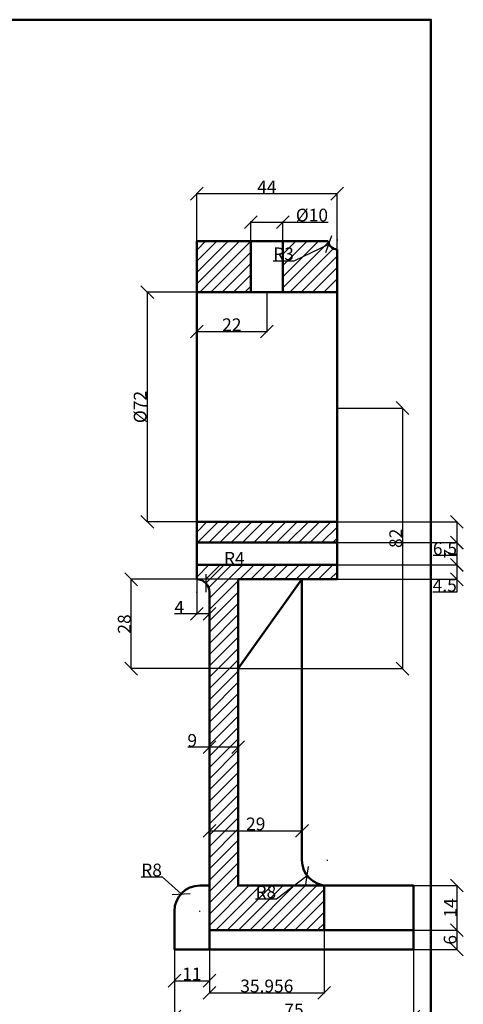
# Model space of a CAD drawing. Units: millimetres. Extents: x -13 to 343, y 323 to 787.
# Tile 3 of 3: x 204 to 343, y 479 to 787. Entities that reach past the tile are written whole.
import ezdxf

# ---------------------------------------------------------------- set-up
doc = ezdxf.new("R2010")
doc.units = ezdxf.units.MM
doc.header["$MEASUREMENT"] = 0
doc.header["$PDMODE"] = 3
doc.header["$PDSIZE"] = -8
for name, color, linetype, lineweight in [('M-DIMS', 2, 'Continuous', 25), ('M-HATC', 8, 'Continuous', 18), ('M-OUTL', 7, 'Continuous', 50), ('M-TTLB', 7, 'Continuous', 50)]:
    doc.layers.add(name, color=color, linetype=linetype, lineweight=lineweight)
doc.styles.get("Standard").update_dxf_attribs({"font": 'arial.ttf'})
doc.dimstyles.get("Standard").update_dxf_attribs({"dimtxt": 4, "dimasz": 4, "dimexe": 0.18, "dimexo": 0.0625, "dimgap": 0.09, "dimtad": 1, "dimtoh": 1, "dimdec": 0, "dimzin": 0, "dimdsep": 46, "dimtxsty": 'Standard', "dimblk": 'OBLIQUE', "dimcen": 0.09, "dimclre": 251, "dimadec": 0, "dimazin": 0, "dimtfac": 1, "dimtdec": 0, "dimtofl": 0, "dimtmove": 0, "dimatfit": 3, "dimfxl": 1, "dimtolj": 1, "dimtzin": 0, "dimarcsym": 0})
pattern_1 = [(45, (-24.6917, 0), (-1.767767, 1.767767), [])]

# ---------------------------------------------------------------- blocks, each defined once
blk = doc.blocks.new('_Oblique')
at = {"color": 0, "linetype": 'ByBlock', "lineweight": -2}
blk.add_line((-0.5, -0.5), (0.5, 0.5), dxfattribs=at)
blk = doc.blocks.new('*D23')
at = {"layer": 'Defpoints', "color": 0, "transparency": 16777216}
for p in [(303.08, 732.78), (259.08, 717.9), (303.08, 715.28)]:
    blk.add_point(p, dxfattribs=at)
at = {"layer": 'M-DIMS', "color": 0, "lineweight": -2, "transparency": 16777216}
for p, q in [((259.08, 717.96), (259.08, 732.96)), ((259.08, 732.78), (303.08, 732.78)), ((303.08, 715.35), (303.08, 732.96))]:
    blk.add_line(p, q, dxfattribs=at)
at = {"layer": 'M-DIMS', "color": 0, "lineweight": -2, "transparency": 16777216, "xscale": 4, "yscale": 4, "zscale": 4, "rotation": 180}
blk.add_blockref('_Oblique', (259.08, 732.78), dxfattribs=at)
at = {"layer": 'M-DIMS', "color": 0, "lineweight": -2, "transparency": 16777216, "xscale": 4, "yscale": 4, "zscale": 4}
blk.add_blockref('_Oblique', (303.08, 732.78), dxfattribs=at)
at = {"layer": 'M-DIMS', "color": 0, "transparency": 16777216, "insert": (281.08, 734.87), "char_height": 4, "attachment_point": 5}
blk.add_mtext('\\A1;44', dxfattribs=at)
blk = doc.blocks.new('*D24')
at = {"layer": 'Defpoints', "color": 0, "transparency": 16777216}
for p in [(286.08, 723.82), (276.08, 717.9), (286.08, 717.9)]:
    blk.add_point(p, dxfattribs=at)
at = {"layer": 'M-DIMS', "color": 0, "lineweight": -2, "transparency": 16777216}
for p, q in [((276.08, 717.96), (276.08, 724)), ((276.08, 723.82), (286.08, 723.82)), ((286.08, 717.96), (286.08, 724)), ((286.08, 723.82), (300.32, 723.82))]:
    blk.add_line(p, q, dxfattribs=at)
at = {"layer": 'M-DIMS', "color": 0, "lineweight": -2, "transparency": 16777216, "xscale": 4, "yscale": 4, "zscale": 4, "rotation": 180}
blk.add_blockref('_Oblique', (276.08, 723.82), dxfattribs=at)
at = {"layer": 'M-DIMS', "color": 0, "lineweight": -2, "transparency": 16777216, "xscale": 4, "yscale": 4, "zscale": 4}
blk.add_blockref('_Oblique', (286.08, 723.82), dxfattribs=at)
at = {"layer": 'M-DIMS', "color": 0, "transparency": 16777216, "insert": (295.2, 726.06), "char_height": 4, "attachment_point": 5}
blk.add_mtext('\\A1;%%C10', dxfattribs=at)
blk = doc.blocks.new('*D25')
at = {"layer": 'Defpoints', "color": 0, "transparency": 16777216}
for p in [(259.08, 701.9), (243.58, 629.9), (259.08, 629.9)]:
    blk.add_point(p, dxfattribs=at)
at = {"layer": 'M-DIMS', "color": 0, "lineweight": -2, "transparency": 16777216}
for p, q in [((259.01, 701.9), (243.4, 701.9)), ((243.58, 701.9), (243.58, 629.9)), ((259.01, 629.9), (243.4, 629.9))]:
    blk.add_line(p, q, dxfattribs=at)
at = {"layer": 'M-DIMS', "color": 0, "lineweight": -2, "transparency": 16777216, "xscale": 4, "yscale": 4, "zscale": 4}
for p, rotation in [((243.58, 701.9), 90), ((243.58, 629.9), 270)]:
    blk.add_blockref('_Oblique', p, dxfattribs=dict(at, rotation=rotation))
at = {"layer": 'M-DIMS', "color": 0, "transparency": 16777216, "insert": (241.33, 665.9), "char_height": 4, "attachment_point": 5, "rotation": 90}
blk.add_mtext('\\A1;%%C72', dxfattribs=at)
blk = doc.blocks.new('*D26')
at = {"layer": 'Defpoints', "color": 0, "transparency": 16777216}
for p in [(259.08, 701.9), (281.08, 701.9), (281.08, 689.59)]:
    blk.add_point(p, dxfattribs=at)
at = {"layer": 'M-DIMS', "color": 0, "lineweight": -2, "transparency": 16777216}
for p, q in [((259.08, 701.83), (259.08, 689.41)), ((281.08, 701.83), (281.08, 689.41)), ((259.08, 689.59), (281.08, 689.59))]:
    blk.add_line(p, q, dxfattribs=at)
at = {"layer": 'M-DIMS', "color": 0, "lineweight": -2, "transparency": 16777216, "xscale": 4, "yscale": 4, "zscale": 4, "rotation": 180}
blk.add_blockref('_Oblique', (259.08, 689.59), dxfattribs=at)
at = {"layer": 'M-DIMS', "color": 0, "lineweight": -2, "transparency": 16777216, "xscale": 4, "yscale": 4, "zscale": 4}
blk.add_blockref('_Oblique', (281.08, 689.59), dxfattribs=at)
at = {"layer": 'M-DIMS', "color": 0, "transparency": 16777216, "insert": (270.08, 691.69), "char_height": 4, "attachment_point": 5}
blk.add_mtext('\\A1;22', dxfattribs=at)
blk = doc.blocks.new('*D27')
at = {"layer": 'Defpoints', "color": 0, "transparency": 16777216}
for p in [(303.08, 665.59), (272.08, 583.9), (323.62, 583.9)]:
    blk.add_point(p, dxfattribs=at)
at = {"layer": 'M-DIMS', "color": 0, "lineweight": -2, "transparency": 16777216}
for p, q in [((303.14, 665.59), (323.8, 665.59)), ((323.62, 665.59), (323.62, 583.9)), ((272.14, 583.9), (323.8, 583.9))]:
    blk.add_line(p, q, dxfattribs=at)
at = {"layer": 'M-DIMS', "color": 0, "lineweight": -2, "transparency": 16777216, "xscale": 4, "yscale": 4, "zscale": 4}
for p, rotation in [((323.62, 665.59), 90), ((323.62, 583.9), 270)]:
    blk.add_blockref('_Oblique', p, dxfattribs=dict(at, rotation=rotation))
at = {"layer": 'M-DIMS', "color": 0, "transparency": 16777216, "insert": (321.49, 624.74), "char_height": 4, "attachment_point": 5, "rotation": 90}
blk.add_mtext('\\A1;82', dxfattribs=at)
blk = doc.blocks.new('*D28')
at = {"layer": 'Defpoints', "color": 0, "transparency": 16777216}
for p in [(259.08, 611.9), (263.08, 601.06), (263.08, 601.06)]:
    blk.add_point(p, dxfattribs=at)
at = {"layer": 'M-DIMS', "color": 0, "lineweight": -2, "transparency": 16777216}
for p, q in [((259.08, 611.83), (259.08, 600.88)), ((259.08, 601.06), (252.13, 601.06)), ((263.08, 601.06), (259.08, 601.06)), ((263.08, 601.12), (263.08, 601.24))]:
    blk.add_line(p, q, dxfattribs=at)
at = {"layer": 'M-DIMS', "color": 0, "lineweight": -2, "transparency": 16777216, "xscale": 4, "yscale": 4, "zscale": 4, "rotation": 180}
blk.add_blockref('_Oblique', (259.08, 601.06), dxfattribs=at)
at = {"layer": 'M-DIMS', "color": 0, "lineweight": -2, "transparency": 16777216, "xscale": 4, "yscale": 4, "zscale": 4}
blk.add_blockref('_Oblique', (263.08, 601.06), dxfattribs=at)
at = {"layer": 'M-DIMS', "color": 0, "transparency": 16777216, "insert": (253.6, 603.15), "char_height": 4, "attachment_point": 5}
blk.add_mtext('\\A1;4', dxfattribs=at)
blk = doc.blocks.new('*D29')
at = {"layer": 'Defpoints', "color": 0, "transparency": 16777216}
for p in [(263.08, 559.26), (263.08, 558.54), (272.08, 558.54)]:
    blk.add_point(p, dxfattribs=at)
at = {"layer": 'M-DIMS', "color": 0, "lineweight": -2, "transparency": 16777216}
for p, q in [((263.08, 559.26), (256.27, 559.26)), ((263.08, 558.6), (263.08, 559.44)), ((272.08, 559.26), (263.08, 559.26)), ((272.08, 558.6), (272.08, 559.44))]:
    blk.add_line(p, q, dxfattribs=at)
at = {"layer": 'M-DIMS', "color": 0, "lineweight": -2, "transparency": 16777216, "xscale": 4, "yscale": 4, "zscale": 4, "rotation": 180}
blk.add_blockref('_Oblique', (263.08, 559.26), dxfattribs=at)
at = {"layer": 'M-DIMS', "color": 0, "lineweight": -2, "transparency": 16777216, "xscale": 4, "yscale": 4, "zscale": 4}
blk.add_blockref('_Oblique', (272.08, 559.26), dxfattribs=at)
at = {"layer": 'M-DIMS', "color": 0, "transparency": 16777216, "insert": (257.67, 561.39), "char_height": 4, "attachment_point": 5}
blk.add_mtext('\\A1;9', dxfattribs=at)
blk = doc.blocks.new('*D30')
at = {"layer": 'Defpoints', "color": 0, "transparency": 16777216}
for p in [(263.08, 533.08), (292.08, 533.08), (292.08, 533.08)]:
    blk.add_point(p, dxfattribs=at)
at = {"layer": 'M-DIMS', "color": 0, "lineweight": -2, "transparency": 16777216}
for p, q in [((263.08, 533.15), (263.08, 533.26)), ((263.08, 533.08), (292.08, 533.08)), ((292.08, 533.15), (292.08, 533.26))]:
    blk.add_line(p, q, dxfattribs=at)
at = {"layer": 'M-DIMS', "color": 0, "lineweight": -2, "transparency": 16777216, "xscale": 4, "yscale": 4, "zscale": 4, "rotation": 180}
blk.add_blockref('_Oblique', (263.08, 533.08), dxfattribs=at)
at = {"layer": 'M-DIMS', "color": 0, "lineweight": -2, "transparency": 16777216, "xscale": 4, "yscale": 4, "zscale": 4}
blk.add_blockref('_Oblique', (292.08, 533.08), dxfattribs=at)
at = {"layer": 'M-DIMS', "color": 0, "transparency": 16777216, "insert": (277.58, 535.22), "char_height": 4, "attachment_point": 5}
blk.add_mtext('\\A1;29', dxfattribs=at)
blk = doc.blocks.new('*D31')
at = {"layer": 'Defpoints', "color": 0, "transparency": 16777216}
for p in [(252.08, 495.9), (263.08, 495.9), (263.08, 486.09)]:
    blk.add_point(p, dxfattribs=at)
at = {"layer": 'M-DIMS', "color": 0, "lineweight": -2, "transparency": 16777216}
for p, q in [((252.08, 495.83), (252.08, 485.91)), ((263.08, 495.83), (263.08, 485.91)), ((252.08, 486.09), (263.08, 486.09))]:
    blk.add_line(p, q, dxfattribs=at)
at = {"layer": 'M-DIMS', "color": 0, "lineweight": -2, "transparency": 16777216, "xscale": 4, "yscale": 4, "zscale": 4, "rotation": 180}
blk.add_blockref('_Oblique', (252.08, 486.09), dxfattribs=at)
at = {"layer": 'M-DIMS', "color": 0, "lineweight": -2, "transparency": 16777216, "xscale": 4, "yscale": 4, "zscale": 4}
blk.add_blockref('_Oblique', (263.08, 486.09), dxfattribs=at)
at = {"layer": 'M-DIMS', "color": 0, "transparency": 16777216, "insert": (257.58, 488.19), "char_height": 4, "attachment_point": 5}
blk.add_mtext('\\A1;11', dxfattribs=at)
blk = doc.blocks.new('*D32')
at = {"layer": 'Defpoints', "color": 0, "transparency": 16777216}
for p in [(252.08, 495.9), (327.08, 495.9), (327.08, 474.82)]:
    blk.add_point(p, dxfattribs=at)
at = {"layer": 'M-DIMS', "color": 0, "lineweight": -2, "transparency": 16777216}
for p, q in [((252.08, 495.83), (252.08, 474.64)), ((327.08, 495.83), (327.08, 474.64)), ((252.08, 474.82), (327.08, 474.82))]:
    blk.add_line(p, q, dxfattribs=at)
at = {"layer": 'M-DIMS', "color": 0, "lineweight": -2, "transparency": 16777216, "xscale": 4, "yscale": 4, "zscale": 4, "rotation": 180}
blk.add_blockref('_Oblique', (252.08, 474.82), dxfattribs=at)
at = {"layer": 'M-DIMS', "color": 0, "lineweight": -2, "transparency": 16777216, "xscale": 4, "yscale": 4, "zscale": 4}
blk.add_blockref('_Oblique', (327.08, 474.82), dxfattribs=at)
at = {"layer": 'M-DIMS', "color": 0, "transparency": 16777216, "insert": (289.58, 476.94), "char_height": 4, "attachment_point": 5}
blk.add_mtext('\\A1;75', dxfattribs=at)
blk = doc.blocks.new('*D57')
at = {"layer": 'Defpoints', "color": 0, "transparency": 16777216}
for p in [(303.08, 629.9), (303.08, 623.4), (340.68, 623.4)]:
    blk.add_point(p, dxfattribs=at)
at = {"layer": 'M-DIMS', "color": 251, "lineweight": -2, "transparency": 16777216}
for p, q in [((303.14, 629.9), (340.86, 629.9)), ((303.14, 623.4), (340.86, 623.4))]:
    blk.add_line(p, q, dxfattribs=at)
at = {"layer": 'M-DIMS', "color": 0, "lineweight": -2, "transparency": 16777216}
for p, q in [((340.68, 629.9), (340.68, 623.4)), ((340.68, 623.4), (340.68, 619.4)), ((340.68, 619.4), (333.25, 619.4))]:
    blk.add_line(p, q, dxfattribs=at)
at = {"layer": 'M-DIMS', "color": 0, "lineweight": -2, "transparency": 16777216, "xscale": 4, "yscale": 4, "zscale": 4}
for p, rotation in [((340.68, 629.9), 90), ((340.68, 623.4), 270)]:
    blk.add_blockref('_Oblique', p, dxfattribs=dict(at, rotation=rotation))
at = {"layer": 'M-DIMS', "color": 0, "transparency": 16777216, "insert": (336.92, 621.53), "char_height": 4, "attachment_point": 5}
blk.add_mtext('\\A1;6.5', dxfattribs=at)
blk = doc.blocks.new('*D58')
at = {"layer": 'Defpoints', "color": 0, "transparency": 16777216}
for p in [(303.076354, 623.396145), (303.076354, 616.396145), (340.676354, 616.396145)]:
    blk.add_point(p, dxfattribs=at)
at = {"layer": 'M-DIMS', "color": 251, "lineweight": -2, "transparency": 16777216}
for p, q in [((303.138854, 623.396145), (340.856354, 623.396145)), ((303.138854, 616.396145), (340.856354, 616.396145))]:
    blk.add_line(p, q, dxfattribs=at)
at = {"layer": 'M-DIMS', "color": 0, "lineweight": -2, "transparency": 16777216}
blk.add_line((340.676354, 623.396145), (340.676354, 616.396145), dxfattribs=at)
at = {"layer": 'M-DIMS', "color": 0, "lineweight": -2, "transparency": 16777216, "xscale": 4, "yscale": 4, "zscale": 4}
for p, rotation in [((340.676354, 623.396145), 90), ((340.676354, 616.396145), 270)]:
    blk.add_blockref('_Oblique', p, dxfattribs=dict(at, rotation=rotation))
at = {"layer": 'M-DIMS', "color": 0, "transparency": 16777216, "insert": (338.586354, 619.896145), "char_height": 4, "attachment_point": 5, "rotation": 90}
blk.add_mtext('\\A1;7', dxfattribs=at)
blk = doc.blocks.new('*D59')
at = {"layer": 'Defpoints', "color": 0, "transparency": 16777216}
for p in [(303.08, 616.4), (303.08, 611.9), (340.68, 611.9)]:
    blk.add_point(p, dxfattribs=at)
at = {"layer": 'M-DIMS', "color": 251, "lineweight": -2, "transparency": 16777216}
for p, q in [((303.14, 616.4), (340.86, 616.4)), ((303.14, 611.9), (340.86, 611.9))]:
    blk.add_line(p, q, dxfattribs=at)
at = {"layer": 'M-DIMS', "color": 0, "lineweight": -2, "transparency": 16777216}
for p, q in [((340.68, 616.4), (340.68, 611.9)), ((340.68, 611.9), (340.68, 607.9)), ((340.68, 607.9), (333.11, 607.9))]:
    blk.add_line(p, q, dxfattribs=at)
at = {"layer": 'M-DIMS', "color": 0, "lineweight": -2, "transparency": 16777216, "xscale": 4, "yscale": 4, "zscale": 4}
for p, rotation in [((340.68, 616.4), 90), ((340.68, 611.9), 270)]:
    blk.add_blockref('_Oblique', p, dxfattribs=dict(at, rotation=rotation))
at = {"layer": 'M-DIMS', "color": 0, "transparency": 16777216, "insert": (336.85, 610.02), "char_height": 4, "attachment_point": 5}
blk.add_mtext('\\A1;4.5', dxfattribs=at)
blk = doc.blocks.new('*D60')
at = {"layer": 'Defpoints', "color": 0, "transparency": 16777216}
for p in [(238.48, 611.9), (272.08, 611.9), (272.08, 583.9)]:
    blk.add_point(p, dxfattribs=at)
at = {"layer": 'M-DIMS', "color": 251, "lineweight": -2, "transparency": 16777216}
for p, q in [((272.01, 611.9), (238.3, 611.9)), ((272.01, 583.9), (238.3, 583.9))]:
    blk.add_line(p, q, dxfattribs=at)
at = {"layer": 'M-DIMS', "color": 0, "lineweight": -2, "transparency": 16777216}
blk.add_line((238.48, 583.9), (238.48, 611.9), dxfattribs=at)
at = {"layer": 'M-DIMS', "color": 0, "lineweight": -2, "transparency": 16777216, "xscale": 4, "yscale": 4, "zscale": 4}
for p, rotation in [((238.48, 611.9), 90), ((238.48, 583.9), 270)]:
    blk.add_blockref('_Oblique', p, dxfattribs=dict(at, rotation=rotation))
at = {"layer": 'M-DIMS', "color": 0, "transparency": 16777216, "insert": (236.34, 597.9), "char_height": 4, "attachment_point": 5, "rotation": 90}
blk.add_mtext('\\A1;28', dxfattribs=at)
blk = doc.blocks.new('*D61')
at = {"layer": 'Defpoints', "color": 0, "transparency": 16777216}
for p in [(327.08, 515.9), (327.08, 501.9), (340.68, 501.9)]:
    blk.add_point(p, dxfattribs=at)
at = {"layer": 'M-DIMS', "color": 251, "lineweight": -2, "transparency": 16777216}
for p, q in [((327.14, 515.9), (340.86, 515.9)), ((327.14, 501.9), (340.86, 501.9))]:
    blk.add_line(p, q, dxfattribs=at)
at = {"layer": 'M-DIMS', "color": 0, "lineweight": -2, "transparency": 16777216}
blk.add_line((340.68, 515.9), (340.68, 501.9), dxfattribs=at)
at = {"layer": 'M-DIMS', "color": 0, "lineweight": -2, "transparency": 16777216, "xscale": 4, "yscale": 4, "zscale": 4}
for p, rotation in [((340.68, 515.9), 90), ((340.68, 501.9), 270)]:
    blk.add_blockref('_Oblique', p, dxfattribs=dict(at, rotation=rotation))
at = {"layer": 'M-DIMS', "color": 0, "transparency": 16777216, "insert": (338.58, 508.9), "char_height": 4, "attachment_point": 5, "rotation": 90}
blk.add_mtext('\\A1;14', dxfattribs=at)
blk = doc.blocks.new('*D62')
at = {"layer": 'Defpoints', "color": 0, "transparency": 16777216}
for p in [(327.08, 501.9), (327.08, 495.9), (340.68, 495.9)]:
    blk.add_point(p, dxfattribs=at)
at = {"layer": 'M-DIMS', "color": 251, "lineweight": -2, "transparency": 16777216}
for p, q in [((327.14, 501.9), (340.86, 501.9)), ((327.14, 495.9), (340.86, 495.9))]:
    blk.add_line(p, q, dxfattribs=at)
at = {"layer": 'M-DIMS', "color": 0, "lineweight": -2, "transparency": 16777216}
blk.add_line((340.68, 501.9), (340.68, 495.9), dxfattribs=at)
at = {"layer": 'M-DIMS', "color": 0, "lineweight": -2, "transparency": 16777216, "xscale": 4, "yscale": 4, "zscale": 4}
for p, rotation in [((340.68, 501.9), 90), ((340.68, 495.9), 270)]:
    blk.add_blockref('_Oblique', p, dxfattribs=dict(at, rotation=rotation))
at = {"layer": 'M-DIMS', "color": 0, "transparency": 16777216, "insert": (338.54, 498.9), "char_height": 4, "attachment_point": 5, "rotation": 90}
blk.add_mtext('\\A1;6', dxfattribs=at)
blk = doc.blocks.new('*D63')
at = {"layer": 'Defpoints', "color": 0, "transparency": 16777216}
for p in [(263.08, 501.9), (299.03, 501.9), (299.03, 482.3)]:
    blk.add_point(p, dxfattribs=at)
at = {"layer": 'M-DIMS', "color": 251, "lineweight": -2, "transparency": 16777216}
for p, q in [((263.08, 501.83), (263.08, 482.12)), ((299.03, 501.83), (299.03, 482.12))]:
    blk.add_line(p, q, dxfattribs=at)
at = {"layer": 'M-DIMS', "color": 0, "lineweight": -2, "transparency": 16777216}
blk.add_line((263.08, 482.3), (299.03, 482.3), dxfattribs=at)
at = {"layer": 'M-DIMS', "color": 0, "lineweight": -2, "transparency": 16777216, "xscale": 4, "yscale": 4, "zscale": 4, "rotation": 180}
blk.add_blockref('_Oblique', (263.08, 482.3), dxfattribs=at)
at = {"layer": 'M-DIMS', "color": 0, "lineweight": -2, "transparency": 16777216, "xscale": 4, "yscale": 4, "zscale": 4}
blk.add_blockref('_Oblique', (299.03, 482.3), dxfattribs=at)
at = {"layer": 'M-DIMS', "color": 0, "transparency": 16777216, "insert": (281.05, 484.43), "char_height": 4, "attachment_point": 5}
blk.add_mtext('\\A1;35.956', dxfattribs=at)
blk = doc.blocks.new('*D74')
at = {"layer": 'Defpoints', "color": 0, "transparency": 16777216}
for p in [(254.15, 513.27), (260.08, 507.9)]:
    blk.add_point(p, dxfattribs=at)
at = {"layer": 'M-DIMS', "color": 0, "lineweight": -2, "transparency": 16777216}
for p, q in [((241.68, 518.65), (248.23, 518.65)), ((248.23, 518.65), (254.15, 513.27))]:
    blk.add_line(p, q, dxfattribs=at)
at = {"layer": 'M-DIMS', "color": 251, "lineweight": -2, "transparency": 16777216}
for p, q in [((259.99, 507.9), (260.17, 507.9)), ((260.08, 507.81), (260.08, 507.99))]:
    blk.add_line(p, q, dxfattribs=at)
at = {"layer": 'M-DIMS', "color": 0, "lineweight": -2, "transparency": 16777216, "xscale": 4, "yscale": 4, "zscale": 4, "rotation": 317.7822941843746}
blk.add_blockref('_Oblique', (254.15, 513.27), dxfattribs=at)
at = {"layer": 'M-DIMS', "color": 0, "transparency": 16777216, "insert": (244.91, 520.78), "char_height": 4, "attachment_point": 5}
blk.add_mtext('\\A1;R8', dxfattribs=at)
blk = doc.blocks.new('*D75')
at = {"layer": 'Defpoints', "color": 0, "transparency": 16777216}
for p in [(261.9, 610.72), (259.08, 607.9)]:
    blk.add_point(p, dxfattribs=at)
at = {"layer": 'M-DIMS', "color": 0, "lineweight": -2, "transparency": 16777216}
for p, q in [((267.56, 616.38), (261.9, 610.72)), ((274.09, 616.38), (267.56, 616.38))]:
    blk.add_line(p, q, dxfattribs=at)
at = {"layer": 'M-DIMS', "color": 251, "lineweight": -2, "transparency": 16777216}
for p, q in [((259.08, 607.81), (259.08, 607.99)), ((258.99, 607.9), (259.17, 607.9))]:
    blk.add_line(p, q, dxfattribs=at)
at = {"layer": 'M-DIMS', "color": 0, "lineweight": -2, "transparency": 16777216, "xscale": 4, "yscale": 4, "zscale": 4, "rotation": 225.0021168684563}
blk.add_blockref('_Oblique', (261.9, 610.72), dxfattribs=at)
at = {"layer": 'M-DIMS', "color": 0, "transparency": 16777216, "insert": (270.87, 618.47), "char_height": 4, "attachment_point": 5}
blk.add_mtext('\\A1;R4', dxfattribs=at)
blk = doc.blocks.new('*D76')
at = {"layer": 'Defpoints', "color": 0, "transparency": 16777216}
for p in [(300.08, 523.9), (293.7, 519.06)]:
    blk.add_point(p, dxfattribs=at)
at = {"layer": 'M-DIMS', "color": 251, "lineweight": -2, "transparency": 16777216}
for p, q in [((299.99, 523.9), (300.17, 523.9)), ((300.08, 523.81), (300.08, 523.99))]:
    blk.add_line(p, q, dxfattribs=at)
at = {"layer": 'M-DIMS', "color": 0, "lineweight": -2, "transparency": 16777216}
for p, q in [((284.07, 511.76), (293.7, 519.06)), ((277.52, 511.76), (284.07, 511.76))]:
    blk.add_line(p, q, dxfattribs=at)
at = {"layer": 'M-DIMS', "color": 0, "lineweight": -2, "transparency": 16777216, "xscale": 4, "yscale": 4, "zscale": 4, "rotation": 37.16993550266607}
blk.add_blockref('_Oblique', (293.7, 519.06), dxfattribs=at)
at = {"layer": 'M-DIMS', "color": 0, "transparency": 16777216, "insert": (280.75, 513.89), "char_height": 4, "attachment_point": 5}
blk.add_mtext('\\A1;R8', dxfattribs=at)
blk = doc.blocks.new('*D77')
at = {"layer": 'Defpoints', "color": 0, "transparency": 16777216}
for p in [(300.51, 716.98), (303.22, 718.28)]:
    blk.add_point(p, dxfattribs=at)
at = {"layer": 'M-DIMS', "color": 0, "lineweight": -2, "transparency": 16777216}
for p, q in [((289.61, 711.77), (300.51, 716.98)), ((283.07, 711.77), (289.61, 711.77))]:
    blk.add_line(p, q, dxfattribs=at)
at = {"layer": 'M-DIMS', "color": 251, "lineweight": -2, "transparency": 16777216}
for p, q in [((303.13, 718.28), (303.31, 718.28)), ((303.22, 718.19), (303.22, 718.37))]:
    blk.add_line(p, q, dxfattribs=at)
at = {"layer": 'M-DIMS', "color": 0, "lineweight": -2, "transparency": 16777216, "xscale": 4, "yscale": 4, "zscale": 4, "rotation": 25.58244592210288}
blk.add_blockref('_Oblique', (300.51, 716.98), dxfattribs=at)
at = {"layer": 'M-DIMS', "color": 0, "transparency": 16777216, "insert": (286.29, 713.9), "char_height": 4, "attachment_point": 5}
blk.add_mtext('\\A1;R3', dxfattribs=at)

msp = doc.modelspace()

# ---------------------------------------------------------------- hatches: boundary and pattern name
at = {"layer": 'M-HATC'}
h = msp.add_hatch(dxfattribs=at)
h.set_pattern_fill('ANSI31', color=256, scale=20)
h.set_pattern_definition(pattern_1)
h.paths.add_polyline_path([(276.0764, 717.8961), (259.0764, 717.8961), (259.0764, 701.8961), (276.0764, 701.8961)])
h.paths.add_polyline_path([(303.0764, 715.2832, -0.36371197), (300.2425, 717.8961), (286.0764, 717.8961), (286.0764, 701.8961), (303.0764, 701.8961)])
h.paths.add_polyline_path([(303.0764, 629.8961), (259.0764, 629.8961), (259.0764, 623.3961), (303.0764, 623.3961)])
h.paths.add_polyline_path([(303.0764, 616.3961), (259.0764, 616.3961), (259.0764, 611.8961), (263.0764, 611.8961), (263.0764, 515.8961), (272.0764, 515.8961), (272.0764, 611.8961), (303.0764, 611.8961)])
h = msp.add_hatch(dxfattribs=at)
h.set_pattern_fill('ANSI31', color=256, scale=20)
h.set_pattern_definition(pattern_1)
h.paths.add_polyline_path([(299.0326, 501.8961), (299.0326, 515.8961), (272.0764, 515.8961), (272.0764, 611.8961), (303.0764, 611.8961), (303.0764, 616.3961), (259.0764, 616.3961), (259.0764, 611.8961), (263.0764, 611.8961), (263.0764, 515.8961), (263.0764, 501.8961)])

# ---------------------------------------------------------------- linework, layer by layer
at = {"layer": 'M-OUTL'}
for p, q in [((259.0764, 611.8961), (259.0764, 717.8961)), ((259.0764, 717.8961), (300.2425, 717.8961)), ((276.0764, 701.8961), (276.0764, 717.8961)), ((286.0764, 701.8961), (286.0764, 717.8961)), ((303.0764, 611.8961), (303.0764, 715.2832)), ((259.0764, 701.8961), (303.0764, 701.8961)), ((259.0764, 629.8961), (303.0764, 629.8961)), ((259.0764, 623.3961), (303.0764, 623.3961)), ((259.0764, 616.3961), (303.0764, 616.3961)), ((259.0764, 611.8961), (259.0764, 611.8961)), ((272.0764, 515.8961), (272.0764, 611.8961)), ((272.0764, 611.8961), (303.0764, 611.8961)), ((292.0764, 611.8961), (272.0764, 583.8961)), ((292.0764, 523.8961), (292.0764, 611.8961)), ((263.0764, 515.8961), (263.0764, 607.8961)), ((263.0764, 515.8961), (260.0764, 515.8961)), ((263.0764, 495.8961), (263.0764, 515.8961)), ((327.0764, 515.8961), (272.0013, 515.8961)), ((299.0326, 515.9645), (299.0326, 501.8961)), ((327.0764, 495.8961), (327.0764, 515.8961)), ((252.0764, 495.8961), (252.0764, 507.8961)), ((263.0764, 501.8961), (327.0764, 501.8961)), ((252.0764, 495.8961), (327.0764, 495.8961))]:
    msp.add_line(p, q, dxfattribs=at)
for centre, radius, start, end in [((303.2178, 718.2799), 3, 187.349107, 267.296837), ((259.0764, 607.8961), 4, 0, 90), ((300.0764, 523.8961), 8, 180, 270), ((260.0764, 507.8961), 8, 90, 180)]:
    msp.add_arc(centre, radius, start, end, dxfattribs=at)
at = {"layer": 'M-TTLB'}
msp.add_lwpolyline([(-13.1348, 787.3025), (332.5007, 787.3025), (332.5007, 323.2082), (-13.1348, 323.2082)], close=True, dxfattribs=at)

# ---------------------------------------------------------------- dimensions: what is measured, and where the dimension line sits
at = {"layer": 'M-DIMS'}
for base, p1, p2, override, picture, middle in [((303.0764, 732.7784), (259.0764, 717.8961), (303.0764, 715.2832), {"dimclrd": 0, "dimclre": 0, "dimclrt": 0}, '*D23', (281.0764, 734.8684)), ((281.0764, 689.5896), (259.0764, 701.8961), (281.0764, 701.8961), {"dimclrd": 0, "dimclre": 0, "dimclrt": 0}, '*D26', (270.0764, 691.6877)), ((292.0764, 533.0841), (263.0764, 533.0841), (292.0764, 533.0841), {"dimclrd": 0, "dimclre": 0, "dimclrt": 0}, '*D30', (277.5764, 535.2164)), ((299.0326, 482.2961), (263.0764, 501.8961), (299.0326, 501.8961), {"dimdec": 3, "dimlfac": 1, "dimrnd": 0, "dimzin": 0, "dimdsep": 46, "dimlunit": 2}, '*D63', (281.0545, 484.4298)), ((263.0764, 486.0942), (252.0764, 495.8961), (263.0764, 495.8961), {"dimclrd": 0, "dimclre": 0, "dimclrt": 0}, '*D31', (257.5764, 488.1923)), ((327.0764, 474.8184), (252.0764, 495.8961), (327.0764, 495.8961), {"dimclrd": 0, "dimclre": 0, "dimclrt": 0}, '*D32', (289.5764, 476.9425))]:
    dim = msp.add_linear_dim(base=base, p1=p1, p2=p2, dimstyle='Standard', override=override, dxfattribs=at)
    dim.commit()
    dim.dimension.update_dxf_attribs({"geometry": picture, "text_midpoint": middle})
dim = msp.add_linear_dim(base=(286.0764, 723.8174), p1=(276.0764, 717.8961), p2=(286.0764, 717.8961), text='%%C<>', dimstyle='Standard', override={"dimclrd": 0, "dimclre": 0, "dimclrt": 0}, dxfattribs=at)
dim.commit()
dim.dimension.update_dxf_attribs({"geometry": '*D24', "text_midpoint": (295.2005, 726.0616)})
for center, mpoint, picture, middle in [((303.2178, 718.2799), (300.5119, 716.9845), '*D77', (286.2945, 713.8987)), ((259.0764, 607.8961), (261.9047, 610.7247), '*D75', (270.8682, 618.4717)), ((260.0764, 507.8961), (254.1516, 513.2717), '*D74', (244.9076, 520.7796)), ((300.0764, 523.8961), (293.7016, 519.0627), '*D76', (280.7528, 513.8937))]:
    dim = msp.add_radius_dim(center=center, mpoint=mpoint, dimstyle='Standard', override={"dimdec": 0, "dimlfac": 1, "dimrnd": 0, "dimzin": 0, "dimdsep": 46, "dimlunit": 2}, dxfattribs=at)
    dim.commit()
    dim.dimension.update_dxf_attribs({"geometry": picture, "text_midpoint": middle})
dim = msp.add_linear_dim(base=(243.5763, 629.8961), p1=(259.0764, 701.8961), p2=(259.0764, 629.8961), angle=90, text='%%C<>', dimstyle='Standard', override={"dimclrd": 0, "dimclre": 0, "dimclrt": 0}, dxfattribs=at)
dim.commit()
dim.dimension.update_dxf_attribs({"geometry": '*D25', "text_midpoint": (241.3322, 665.8961)})
for base, p1, p2, override, picture, middle in [((323.6185, 583.8961), (303.0764, 665.5897), (272.0764, 583.8961), {"dimclrd": 0, "dimclre": 0, "dimclrt": 0}, '*D27', (321.4862, 624.7429)), ((340.6764, 623.3961), (303.0764, 629.8961), (303.0764, 623.3961), {"dimdec": 1, "dimlfac": 1, "dimrnd": 0, "dimzin": 0, "dimdsep": 46, "dimlunit": 2}, '*D57', (336.9192, 621.5284)), ((340.6764, 616.3961), (303.0764, 623.3961), (303.0764, 616.3961), {"dimdec": 0, "dimlfac": 1, "dimrnd": 0, "dimzin": 0, "dimdsep": 46, "dimlunit": 2}, '*D58', (338.5864, 619.8961)), ((340.6764, 611.8961), (303.0764, 616.3961), (303.0764, 611.8961), {"dimdec": 1, "dimlfac": 1, "dimrnd": 0, "dimzin": 0, "dimdsep": 46, "dimlunit": 2}, '*D59', (336.8497, 610.0203)), ((238.4764, 611.8961), (272.0764, 583.8961), (272.0764, 611.8961), {"dimdec": 0, "dimlfac": 1, "dimrnd": 0, "dimzin": 0, "dimdsep": 46, "dimlunit": 2}, '*D60', (236.3441, 597.8961)), ((340.6764, 501.8961), (327.0764, 515.8961), (327.0764, 501.8961), {"dimdec": 0, "dimlfac": 1, "dimrnd": 0, "dimzin": 0, "dimdsep": 46, "dimlunit": 2}, '*D61', (338.5782, 508.8961)), ((340.6764, 495.8961), (327.0764, 501.8961), (327.0764, 495.8961), {"dimdec": 0, "dimlfac": 1, "dimrnd": 0, "dimzin": 0, "dimdsep": 46, "dimlunit": 2}, '*D62', (338.5441, 498.8961))]:
    dim = msp.add_linear_dim(base=base, p1=p1, p2=p2, angle=90, dimstyle='Standard', override=override, dxfattribs=at)
    dim.commit()
    dim.dimension.update_dxf_attribs({"geometry": picture, "text_midpoint": middle})
for base, p1, p2, picture, middle in [((263.0764, 601.0555), (259.0764, 611.8961), (263.0764, 601.0555), '*D28', (253.603, 601.0555)), ((263.0764, 559.2625), (272.0764, 558.5424), (263.0764, 558.5424), '*D29', (257.6712, 559.2625))]:
    dim = msp.add_linear_dim(base=base, p1=p1, p2=p2, dimstyle='Standard', override={"dimclrd": 0, "dimclre": 0, "dimclrt": 0}, dxfattribs=at)
    dim.commit()
    dim.dimension.update_dxf_attribs({"geometry": picture, "text_midpoint": middle, "dimtype": 160})

doc.saveas('drawing.dxf')
